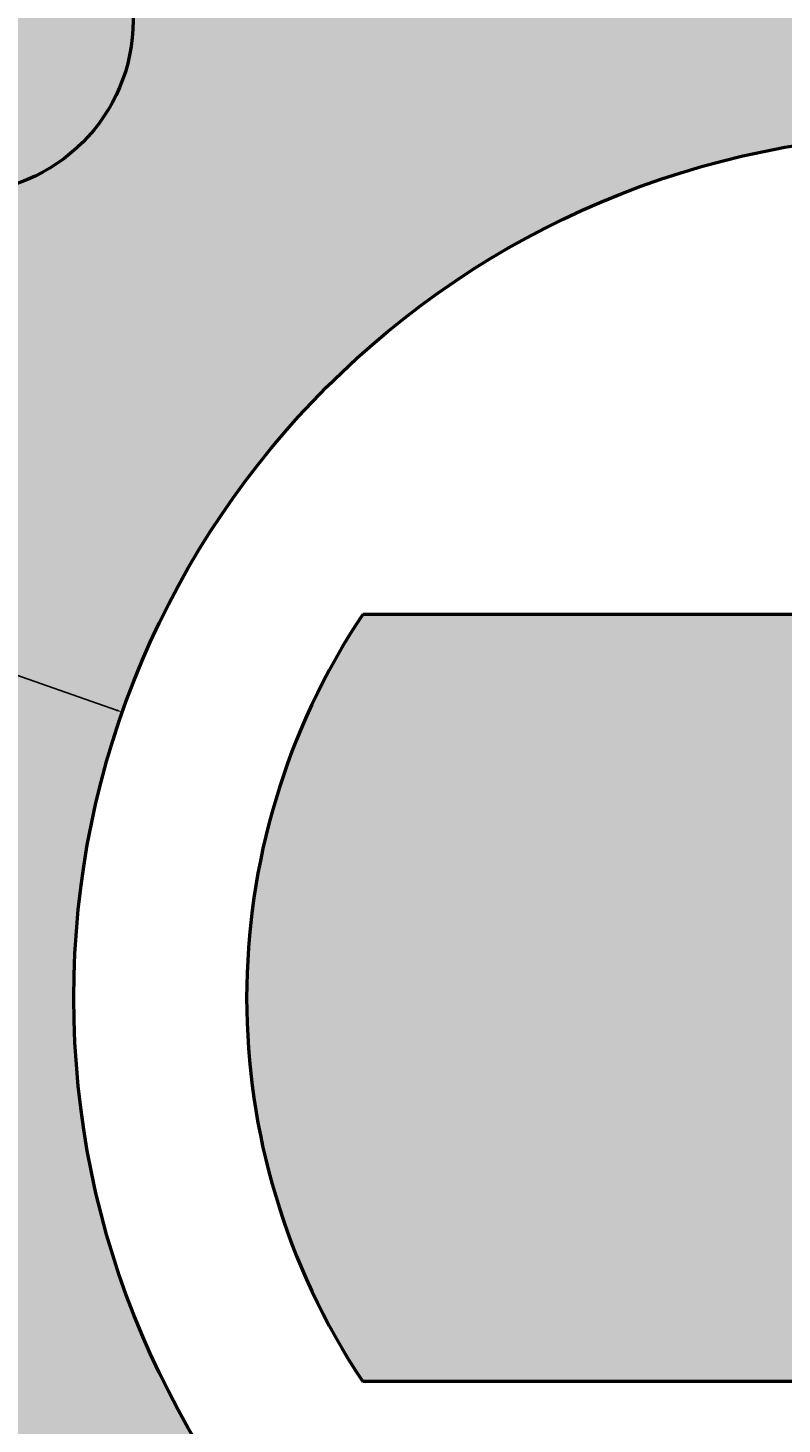
# Model space of a CAD drawing. Units: inches. Extents: x 139261 to 139415, y 52839 to 52963.
# Tile 13 of 20: x 139314 to 139336, y 52888 to 52928. Entities that reach past the tile are written whole.
import ezdxf

# ---------------------------------------------------------------- set-up
doc = ezdxf.new("R2010")
doc.units = ezdxf.units.IN
doc.header["$MEASUREMENT"] = 0
for name, color, linetype, lineweight in [('M-DIMS', 2, 'Continuous', 25), ('M-HATC', 8, 'Continuous', 18), ('M-OUTL', 7, 'Continuous', 50)]:
    doc.layers.add(name, color=color, linetype=linetype, lineweight=lineweight)
doc.styles.get("Standard").update_dxf_attribs({"font": 'arial.ttf'})
doc.dimstyles.get("Standard").update_dxf_attribs({"dimtxt": 0.18, "dimasz": 0.18, "dimexe": 0.18, "dimexo": 0.0625, "dimgap": 0.09, "dimtad": 0, "dimtih": 1, "dimtoh": 1, "dimdec": 4, "dimzin": 0, "dimdsep": 46, "dimtxsty": 'Standard', "dimcen": 0.09, "dimadec": 0, "dimazin": 0, "dimtfac": 1, "dimtdec": 4, "dimtofl": 0, "dimtmove": 0, "dimatfit": 3, "dimfxl": 1, "dimtolj": 1, "dimtzin": 0, "dimarcsym": 0})

# ---------------------------------------------------------------- blocks, each defined once
blk = doc.blocks.new('*U1')
blk.add_circle((0, 0), 5)
blk = doc.blocks.new('*U2')
at = {"layer": 'M-OUTL', "color": 0, "linetype": 'ByBlock', "lineweight": -2, "transparency": 16777216, "rotation": 45.00000000000001}
blk.add_blockref('*U1', (139312.073, 52928.502), dxfattribs=at)
blk = doc.blocks.new('*D3')
at = {"layer": 'Defpoints', "color": 0, "transparency": 16777216}
for p in [(139359.484, 52906.062), (139321.23, 52894.373)]:
    blk.add_point(p, dxfattribs=at)
at = {"layer": 'M-DIMS', "color": 0, "lineweight": -2, "transparency": 16777216}
for p, q in [((139412.091, 52922.136), (139359.656, 52906.115)), ((139412.271, 52922.136), (139412.091, 52922.136)), ((139340.357, 52900.127), (139340.357, 52900.307)), ((139340.267, 52900.217), (139340.447, 52900.217))]:
    blk.add_line(p, q, dxfattribs=at)
at = {"layer": 'M-DIMS', "color": 0, "transparency": 16777216}
blk.add_solid([(139359.647, 52906.143), (139359.665, 52906.086), (139359.484, 52906.062)], dxfattribs=at)
at = {"layer": 'M-DIMS', "color": 0, "transparency": 16777216, "insert": (139412.902, 52922.136), "char_height": 0.18, "attachment_point": 5}
blk.add_mtext('\\A1;∅40.0000', dxfattribs=at)
blk = doc.blocks.new('*D4')
at = {"layer": 'Defpoints', "color": 0, "transparency": 16777216}
for p in [(139373.053, 52923.26), (139307.661, 52877.175)]:
    blk.add_point(p, dxfattribs=at)
at = {"layer": 'M-DIMS', "color": 0, "lineweight": -2, "transparency": 16777216}
for p, q in [((139414.011, 52952.126), (139373.2, 52923.364)), ((139414.191, 52952.126), (139414.011, 52952.126)), ((139340.357, 52900.127), (139340.357, 52900.307)), ((139340.267, 52900.217), (139340.447, 52900.217))]:
    blk.add_line(p, q, dxfattribs=at)
blk.add_arc((139340.357, 52900.217), 40, 34.9168, 52.0771, dxfattribs=at)
at = {"layer": 'M-DIMS', "color": 0, "transparency": 16777216}
blk.add_solid([(139373.183, 52923.388), (139373.217, 52923.339), (139373.053, 52923.26)], dxfattribs=at)
at = {"layer": 'M-DIMS', "color": 0, "transparency": 16777216, "insert": (139414.822, 52952.126), "char_height": 0.18, "attachment_point": 5}
blk.add_mtext('\\A1;∅80.0000', dxfattribs=at)
blk = doc.blocks.new('*D5')
at = {"layer": 'Defpoints', "color": 0, "transparency": 16777216}
for p in [(139316.763, 52908.484), (139363.951, 52891.951)]:
    blk.add_point(p, dxfattribs=at)
at = {"layer": 'M-DIMS', "color": 0, "lineweight": -2, "transparency": 16777216}
for p, q in [((139262.553, 52927.414), (139262.733, 52927.414)), ((139262.733, 52927.414), (139316.593, 52908.544)), ((139340.357, 52900.127), (139340.357, 52900.307)), ((139340.267, 52900.217), (139340.447, 52900.217))]:
    blk.add_line(p, q, dxfattribs=at)
at = {"layer": 'M-DIMS', "color": 0, "transparency": 16777216}
blk.add_solid([(139316.603, 52908.572), (139316.583, 52908.515), (139316.763, 52908.484)], dxfattribs=at)
at = {"layer": 'M-DIMS', "color": 0, "transparency": 16777216, "insert": (139261.922, 52927.414), "char_height": 0.18, "attachment_point": 5}
blk.add_mtext('\\A1;∅50.0000', dxfattribs=at)
blk = doc.blocks.new('*D6')
at = {"layer": 'Defpoints', "color": 0, "transparency": 16777216}
for p in [(139332.153, 52949.54), (139348.561, 52850.895)]:
    blk.add_point(p, dxfattribs=at)
at = {"layer": 'M-DIMS', "color": 0, "lineweight": -2, "transparency": 16777216}
for p, q in [((139329.787, 52962.682), (139329.967, 52962.682)), ((139329.967, 52962.682), (139332.124, 52949.717)), ((139340.357, 52900.127), (139340.357, 52900.307)), ((139340.267, 52900.217), (139340.447, 52900.217))]:
    blk.add_line(p, q, dxfattribs=at)
at = {"layer": 'M-DIMS', "color": 0, "transparency": 16777216}
blk.add_solid([(139332.153, 52949.722), (139332.094, 52949.713), (139332.153, 52949.54)], dxfattribs=at)
at = {"layer": 'M-DIMS', "color": 0, "transparency": 16777216, "insert": (139329.086, 52962.682), "char_height": 0.18, "attachment_point": 5}
blk.add_mtext('\\A1;∅100.0000', dxfattribs=at)
blk = doc.blocks.new('*D9')
at = {"layer": 'Defpoints', "color": 0, "transparency": 16777216}
for p in [(139302.054, 52932.357), (139378.659, 52868.078)]:
    blk.add_point(p, dxfattribs=at)
at = {"layer": 'M-DIMS', "color": 0, "lineweight": -2, "transparency": 16777216}
for p, q in [((139278.893, 52951.64), (139279.073, 52951.64)), ((139279.073, 52951.64), (139301.916, 52932.472)), ((139340.357, 52900.127), (139340.357, 52900.307)), ((139340.267, 52900.217), (139340.447, 52900.217))]:
    blk.add_line(p, q, dxfattribs=at)
at = {"layer": 'M-DIMS', "color": 0, "transparency": 16777216}
blk.add_solid([(139301.936, 52932.495), (139301.897, 52932.449), (139302.054, 52932.357)], dxfattribs=at)
at = {"layer": 'M-DIMS', "color": 0, "transparency": 16777216, "insert": (139278.506, 52951.64), "char_height": 0.18, "attachment_point": 5}
blk.add_mtext('\\A1;∅100', dxfattribs=at)
blk = doc.blocks.new('*D10')
at = {"layer": 'Defpoints', "color": 0, "transparency": 16777216}
for p in [(139325.07, 52937.181), (139355.644, 52863.254)]:
    blk.add_point(p, dxfattribs=at)
at = {"layer": 'M-DIMS', "color": 0, "lineweight": -2, "transparency": 16777216}
for p, q in [((139340.357, 52900.127), (139340.357, 52900.307)), ((139340.267, 52900.217), (139340.447, 52900.217)), ((139364.816, 52841.075), (139355.712, 52863.087)), ((139364.996, 52841.075), (139364.816, 52841.075))]:
    blk.add_line(p, q, dxfattribs=at)
at = {"layer": 'M-DIMS', "color": 0, "transparency": 16777216}
blk.add_solid([(139355.74, 52863.099), (139355.685, 52863.076), (139355.644, 52863.254)], dxfattribs=at)
at = {"layer": 'M-DIMS', "color": 0, "transparency": 16777216, "insert": (139365.312, 52841.075), "char_height": 0.18, "attachment_point": 5}
blk.add_mtext('\\A1;∅80', dxfattribs=at)

msp = doc.modelspace()

# ---------------------------------------------------------------- hatches: boundary and pattern name
at = {"layer": 'M-HATC'}
h = msp.add_hatch(color=256, dxfattribs=at)
h.dxf.hatch_style = 1
h.paths.add_polyline_path([(139290.35689, 52900.21749, 1), (139390.35689, 52900.21749, 1)])
h.paths.add_polyline_path([(139335.36666, 52939.90499, -0.01563646), (139335.35689, 52940.21749, -1), (139345.35689, 52940.21749, -0.01563646), (139345.34711, 52939.90499, -0.13461315), (139364.89157, 52931.80941, -0.691035), (139373.64116, 52928.50176, -0.21521822), (139371.94881, 52924.75216, -0.13461315), (139380.04439, 52905.20771, -0.43265224), (139385.35689, 52900.21749, -0.43265224), (139380.04439, 52895.22726, -0.13461315), (139371.94881, 52875.68281, -0.21521822), (139373.64116, 52871.93321, -0.691035), (139364.89157, 52868.62556, -0.13461315), (139345.34711, 52860.52999, -0.01563646), (139345.35689, 52860.21749, -1), (139335.35689, 52860.21749, -0.01563646), (139335.36666, 52860.52999, -0.13461315), (139315.82221, 52868.62556, -0.691035), (139307.07262, 52871.93321, -0.21521822), (139308.76496, 52875.68281, -0.13461315), (139300.66939, 52895.22726, -0.43265224), (139295.35689, 52900.21749, -0.43265224), (139300.66939, 52905.20771, -0.13461315), (139308.76496, 52924.75216, -0.21521822), (139307.07262, 52928.50176, -0.691035), (139315.82221, 52931.80941, -0.13461315)], flags=16)
h.paths.add_polyline_path([(139365.35689, 52900.21749, -1), (139315.35689, 52900.21749, -1)], flags=0)
h.paths.add_polyline_path([(139323.71474, 52911.30978), (139356.99903, 52911.30978, -0.3027197), (139356.99903, 52889.12519), (139323.71474, 52889.12519, -0.3027197)], flags=0)
h.paths.add_polyline_path([(139364.89157, 52931.80941, 0.13461315), (139345.34711, 52939.90499, -0.93933644), (139335.36666, 52939.90499, 0.13461315), (139315.82221, 52931.80941, -0.18270763), (139317.07262, 52928.50176, -0.64579494), (139308.76496, 52924.75216, 0.13461315), (139300.66939, 52905.20771, -0.39601219), (139305.35689, 52900.21749, -0.39601219), (139300.66939, 52895.22726, 0.13461315), (139308.76496, 52875.68281, -0.64579494), (139317.07262, 52871.93321, -0.18270763), (139315.82221, 52868.62556, 0.13461315), (139335.36666, 52860.52999, -0.93933644), (139345.34711, 52860.52999, 0.13461315), (139364.89157, 52868.62556, -0.18270763), (139363.64116, 52871.93321, -0.64579494), (139371.94881, 52875.68281, 0.13461315), (139380.04439, 52895.22726, -0.39601219), (139375.35689, 52900.21749, -0.39601219), (139380.04439, 52905.20771, 0.13461315), (139371.94881, 52924.75216, -0.64579494), (139363.64116, 52928.50176, -0.18270763)], flags=0)
h = msp.add_hatch(color=256, dxfattribs=at)
h.dxf.hatch_style = 1
h.set_gradient(color1=(205, 105, 40), tint=1)
h.paths.add_polyline_path([(139335.35689, 52940.21749, 1), (139345.35689, 52940.21749, 1)])
h.paths.add_polyline_path([(139307.07262, 52928.50176, 1), (139317.07262, 52928.50176, 1)])
h.paths.add_polyline_path([(139295.35689, 52900.21749, 1), (139305.35689, 52900.21749, 1)])
h.paths.add_polyline_path([(139307.07262, 52871.93321, 1), (139317.07262, 52871.93321, 1)])
h.paths.add_polyline_path([(139345.35689, 52860.21749, 1), (139335.35689, 52860.21749, 1)])
h.paths.add_polyline_path([(139363.64116, 52871.93321, 1), (139373.64116, 52871.93321, 1)])
h.paths.add_polyline_path([(139375.35689, 52900.21749, 1), (139385.35689, 52900.21749, 1)])
h.paths.add_polyline_path([(139363.64116, 52928.50176, 1), (139373.64116, 52928.50176, 1)])
h = msp.add_hatch(color=256, dxfattribs=at)
h.dxf.hatch_style = 1
h.paths.add_polyline_path([(139345.34711, 52939.90499, -0.93933644), (139335.36666, 52939.90499, 0.13461315), (139315.82221, 52931.80941, -0.18270763), (139317.07262, 52928.50176, -0.64579494), (139308.76496, 52924.75216, 0.13461315), (139300.66939, 52905.20771, -0.39601219), (139305.35689, 52900.21749, -0.39601219), (139300.66939, 52895.22726, 0.13461315), (139308.76496, 52875.68281, -0.64579494), (139317.07262, 52871.93321, -0.18270763), (139315.82221, 52868.62556, 0.13461315), (139335.36666, 52860.52999, -0.93933644), (139345.34711, 52860.52999, 0.13461315), (139364.89157, 52868.62556, -0.18270763), (139363.64116, 52871.93321, -0.64579494), (139371.94881, 52875.68281, 0.13461315), (139380.04439, 52895.22726, -0.39601219), (139375.35689, 52900.21749, -0.39601219), (139380.04439, 52905.20771, 0.13461315), (139371.94881, 52924.75216, -0.64579494), (139363.64116, 52928.50176, -0.18270763), (139364.89157, 52931.80941, 0.13461315)])
h.paths.add_polyline_path([(139365.35689, 52900.21749, -1), (139315.35689, 52900.21749, -1)], flags=16)
h.paths.add_polyline_path([(139356.99903, 52911.30978, -0.3027197), (139356.99903, 52889.12519), (139323.71474, 52889.12519, -0.3027197), (139323.71474, 52911.30978)], flags=0)
h = msp.add_hatch(color=256, dxfattribs=at)
h.dxf.hatch_style = 1
h.paths.add_polyline_path([(139356.99903, 52911.30978), (139323.71474, 52911.30978, 0.3027197), (139323.71474, 52889.12519), (139356.99903, 52889.12519, 0.3027197)])

# ---------------------------------------------------------------- linework, layer by layer
at = {"layer": 'M-OUTL'}
for p, q in [((139356.99903, 52911.30978), (139323.71474, 52911.30978)), ((139356.99903, 52889.12519), (139323.71474, 52889.12519))]:
    msp.add_line(p, q, dxfattribs=at)
for radius in [50, 25]:
    msp.add_circle((139340.35689, 52900.21749), radius, dxfattribs=at)
msp.add_arc((139340.35689, 52900.21749), 20, 146.315805, 213.684195, dxfattribs=at)

# ---------------------------------------------------------------- block references
msp.add_blockref('*U2', (0, 0), dxfattribs=at)

# ---------------------------------------------------------------- dimensions: what is measured, and where the dimension line sits
at = {"layer": 'M-DIMS'}
for p1, p2, override, picture, middle in [((139348.56051, 52850.89507), (139332.15326, 52949.5399), {"dimclrd": 0, "dimclre": 0, "dimclrt": 0}, '*D6', (139329.08622, 52962.68242)), ((139307.66087, 52877.17469), (139373.0529, 52923.26028), {"dimclrd": 0, "dimclre": 0, "dimclrt": 0}, '*D4', (139414.82217, 52952.12585)), ((139378.65939, 52868.07845), (139302.05438, 52932.35652), {"dimdec": 0, "dimlfac": 1, "dimrnd": 0, "dimzin": 0, "dimdsep": 46, "dimlunit": 2}, '*D9', (139278.50641, 52951.63995)), ((139325.07023, 52937.18123), (139355.64354, 52863.25374), {"dimdec": 0, "dimlfac": 1, "dimrnd": 0, "dimzin": 0, "dimdsep": 46, "dimlunit": 2}, '*D10', (139365.31206, 52841.0755)), ((139363.95063, 52891.95098), (139316.76314, 52908.48399), {"dimclrd": 0, "dimclre": 0, "dimclrt": 0}, '*D5', (139261.92224, 52927.41429)), ((139321.22987, 52894.37307), (139359.4839, 52906.0619), {"dimclrd": 0, "dimclre": 0, "dimclrt": 0}, '*D3', (139412.90184, 52922.13633))]:
    dim = msp.add_diameter_dim_2p(p1=p1, p2=p2, dimstyle='Standard', override=override, dxfattribs=at)
    dim.commit()
    dim.dimension.update_dxf_attribs({"geometry": picture, "text_midpoint": middle, "dimtype": 163})

doc.saveas('drawing.dxf')
